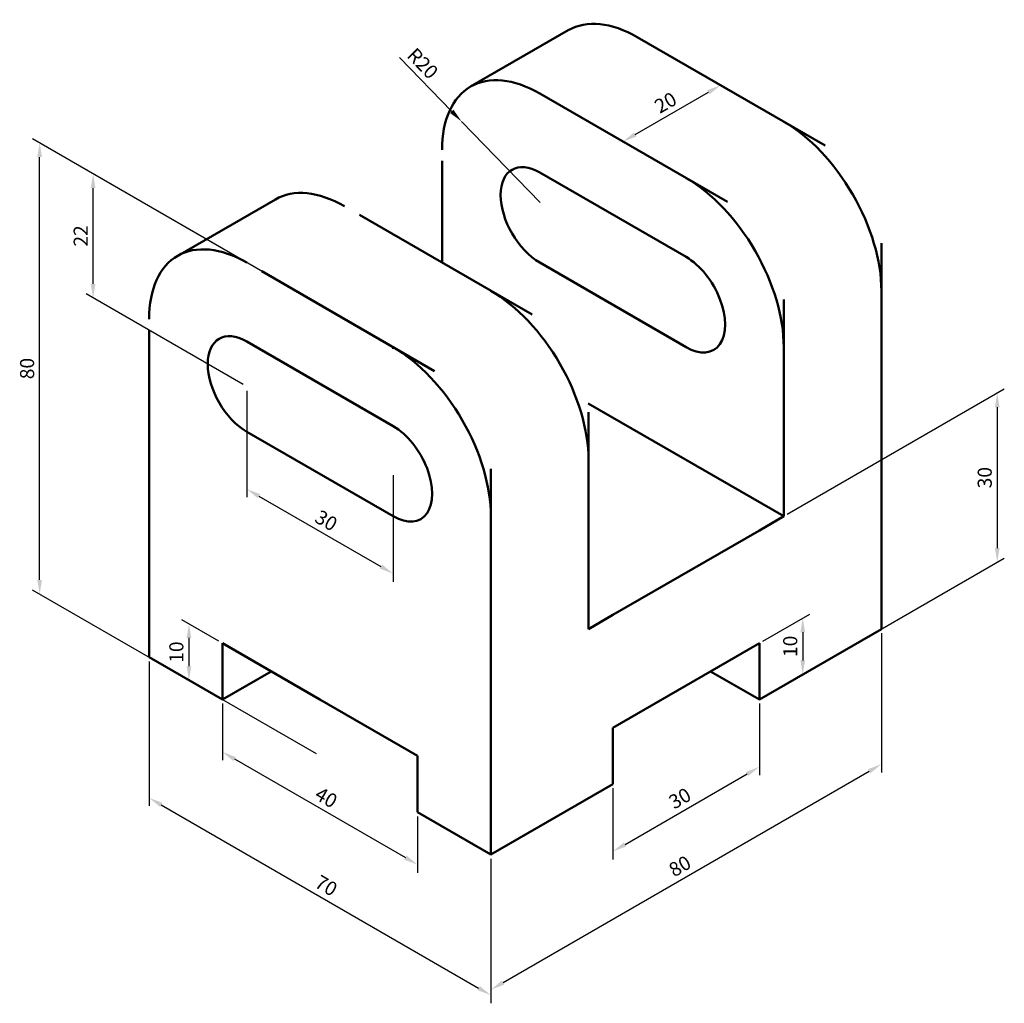
# Model space of a CAD drawing. Units: millimetres. Extents: x 2392 to 2567, y 1870 to 2044.
import ezdxf

# ---------------------------------------------------------------- set-up
doc = ezdxf.new("R2010")
doc.units = ezdxf.units.MM
doc.layers.add('M-DIMS', color=2, linetype='Continuous', lineweight=25)
doc.layers.add('M-OUTL', color=7, linetype='Continuous', lineweight=50)
doc.styles.get("Standard").update_dxf_attribs({"font": 'arial.ttf'})
doc.dimstyles.new('ISO-25', dxfattribs={"dimtxt": 2.5, "dimasz": 2.5, "dimexe": 1.25, "dimexo": 0.625, "dimtad": 1, "dimtxsty": 'Standard', "dimcen": 2.5, "dimadec": 0, "dimazin": 0, "dimtfac": 1, "dimtmove": 0, "dimatfit": 3, "dimfxl": 1, "dimarcsym": 0})

# ---------------------------------------------------------------- blocks, each defined once
blk = doc.blocks.new('*D1')
at = {"layer": 'Defpoints', "color": 0, "transparency": 16777216}
for p in [(2523.54, 1923.45), (2523.54, 1911.51), (2497.56, 1908.45)]:
    blk.add_point(p, dxfattribs=at)
at = {"layer": 'M-DIMS', "color": 0, "lineweight": -2, "transparency": 16777216}
for p, q in [((2523.54, 1922.73), (2523.54, 1910.07)), ((2499.73, 1897.76), (2521.38, 1910.26)), ((2497.56, 1907.73), (2497.56, 1895.07))]:
    blk.add_line(p, q, dxfattribs=at)
at = {"layer": 'M-DIMS', "color": 0, "transparency": 16777216}
for points in [[(2521.17, 1910.62), (2521.58, 1909.9), (2523.54, 1911.51)], [(2499.52, 1898.12), (2499.93, 1897.4), (2497.56, 1896.51)]]:
    blk.add_solid(points, dxfattribs=at)
at = {"layer": 'M-DIMS', "color": 0, "transparency": 16777216, "insert": (2509.6, 1905.66), "char_height": 2.5, "attachment_point": 5, "rotation": 30}
blk.add_mtext('30', dxfattribs=at)
blk = doc.blocks.new('*D2')
at = {"layer": 'Defpoints', "color": 0, "transparency": 16777216}
for p in [(2545.19, 1935.95), (2545.19, 1911.99), (2475.91, 1895.95)]:
    blk.add_point(p, dxfattribs=at)
at = {"layer": 'M-DIMS', "color": 0, "lineweight": -2, "transparency": 16777216}
for p, q in [((2545.19, 1935.23), (2545.19, 1910.54)), ((2478.08, 1873.24), (2543.03, 1910.74)), ((2475.91, 1895.23), (2475.91, 1870.54))]:
    blk.add_line(p, q, dxfattribs=at)
at = {"layer": 'M-DIMS', "color": 0, "transparency": 16777216}
for points in [[(2542.82, 1911.1), (2543.24, 1910.38), (2545.19, 1911.99)], [(2477.87, 1873.6), (2478.28, 1872.88), (2475.91, 1871.99)]]:
    blk.add_solid(points, dxfattribs=at)
at = {"layer": 'M-DIMS', "color": 0, "transparency": 16777216, "insert": (2509.6, 1893.63), "char_height": 2.5, "attachment_point": 5, "rotation": 30}
blk.add_mtext('80', dxfattribs=at)
blk = doc.blocks.new('*D3')
at = {"layer": 'Defpoints', "color": 0, "transparency": 16777216}
for p in [(2428.28, 1923.45), (2462.92, 1903.45), (2462.92, 1894.16)]:
    blk.add_point(p, dxfattribs=at)
at = {"layer": 'M-DIMS', "color": 0, "lineweight": -2, "transparency": 16777216}
for p, q in [((2428.28, 1922.73), (2428.28, 1912.72)), ((2430.44, 1912.91), (2460.75, 1895.41)), ((2462.92, 1902.73), (2462.92, 1892.72))]:
    blk.add_line(p, q, dxfattribs=at)
at = {"layer": 'M-DIMS', "color": 0, "transparency": 16777216}
for points in [[(2430.65, 1913.27), (2430.24, 1912.55), (2428.28, 1914.16)], [(2460.96, 1895.77), (2460.55, 1895.05), (2462.92, 1894.16)]]:
    blk.add_solid(points, dxfattribs=at)
at = {"layer": 'M-DIMS', "color": 0, "transparency": 16777216, "insert": (2446.55, 1905.81), "char_height": 2.5, "attachment_point": 5, "rotation": 330}
blk.add_mtext('40', dxfattribs=at)
blk = doc.blocks.new('*D4')
at = {"layer": 'Defpoints', "color": 0, "transparency": 16777216}
for p in [(2415.29, 1930.95), (2475.91, 1895.95), (2475.91, 1871.02)]:
    blk.add_point(p, dxfattribs=at)
at = {"layer": 'M-DIMS', "color": 0, "lineweight": -2, "transparency": 16777216}
for p, q in [((2415.29, 1930.23), (2415.29, 1904.58)), ((2417.45, 1904.77), (2473.74, 1872.27)), ((2475.91, 1895.23), (2475.91, 1869.58))]:
    blk.add_line(p, q, dxfattribs=at)
at = {"layer": 'M-DIMS', "color": 0, "transparency": 16777216}
for points in [[(2417.66, 1905.13), (2417.24, 1904.41), (2415.29, 1906.02)], [(2473.95, 1872.63), (2473.54, 1871.91), (2475.91, 1871.02)]]:
    blk.add_solid(points, dxfattribs=at)
at = {"layer": 'M-DIMS', "color": 0, "transparency": 16777216, "insert": (2446.55, 1890.17), "char_height": 2.5, "attachment_point": 5, "rotation": 330}
blk.add_mtext('70', dxfattribs=at)
blk = doc.blocks.new('*D5')
at = {"layer": 'Defpoints', "color": 0, "transparency": 16777216}
for p in [(2395.87, 2022.16), (2445.6, 1993.45), (2445.6, 1913.45)]:
    blk.add_point(p, dxfattribs=at)
at = {"layer": 'M-DIMS', "color": 0, "lineweight": -2, "transparency": 16777216}
for p, q in [((2444.97, 1993.81), (2394.62, 2022.88)), ((2395.87, 1944.66), (2395.87, 2019.66)), ((2444.97, 1913.81), (2394.62, 1942.88))]:
    blk.add_line(p, q, dxfattribs=at)
at = {"layer": 'M-DIMS', "color": 0, "transparency": 16777216}
for points in [[(2395.46, 2019.66), (2396.29, 2019.66), (2395.87, 2022.16)], [(2395.46, 1944.66), (2396.29, 1944.66), (2395.87, 1942.16)]]:
    blk.add_solid(points, dxfattribs=at)
at = {"layer": 'M-DIMS', "color": 0, "transparency": 16777216, "insert": (2393.97, 1982.16), "char_height": 2.5, "attachment_point": 5, "rotation": 90}
blk.add_mtext('80', dxfattribs=at)
blk = doc.blocks.new('*D6')
at = {"layer": 'Defpoints', "color": 0, "transparency": 16777216}
for p in [(2405.35, 2016.68), (2432.61, 2000.95), (2432.61, 1978.95)]:
    blk.add_point(p, dxfattribs=at)
at = {"layer": 'M-DIMS', "color": 0, "lineweight": -2, "transparency": 16777216}
for p, q in [((2431.98, 2001.31), (2404.1, 2017.41)), ((2405.35, 1997.18), (2405.35, 2014.18)), ((2431.98, 1979.31), (2404.1, 1995.41))]:
    blk.add_line(p, q, dxfattribs=at)
at = {"layer": 'M-DIMS', "color": 0, "transparency": 16777216}
for points in [[(2404.94, 2014.18), (2405.77, 2014.18), (2405.35, 2016.68)], [(2404.94, 1997.18), (2405.77, 1997.18), (2405.35, 1994.68)]]:
    blk.add_solid(points, dxfattribs=at)
at = {"layer": 'M-DIMS', "color": 0, "transparency": 16777216, "insert": (2403.47, 2005.68), "char_height": 2.5, "attachment_point": 5, "rotation": 90}
blk.add_mtext('22', dxfattribs=at)
blk = doc.blocks.new('*D7')
at = {"layer": 'Defpoints', "color": 0, "transparency": 16777216}
for p in [(2432.61, 1978.95), (2458.59, 1963.95), (2458.59, 1945.78)]:
    blk.add_point(p, dxfattribs=at)
at = {"layer": 'M-DIMS', "color": 0, "lineweight": -2, "transparency": 16777216}
for p, q in [((2432.61, 1978.23), (2432.61, 1959.34)), ((2458.59, 1963.23), (2458.59, 1944.34)), ((2434.77, 1959.53), (2456.42, 1947.03))]:
    blk.add_line(p, q, dxfattribs=at)
at = {"layer": 'M-DIMS', "color": 0, "transparency": 16777216}
for points in [[(2434.98, 1959.89), (2434.57, 1959.17), (2432.61, 1960.78)], [(2456.63, 1947.39), (2456.22, 1946.67), (2458.59, 1945.78)]]:
    blk.add_solid(points, dxfattribs=at)
at = {"layer": 'M-DIMS', "color": 0, "transparency": 16777216, "insert": (2446.55, 1954.93), "char_height": 2.5, "attachment_point": 5, "rotation": 330}
blk.add_mtext('30', dxfattribs=at)
blk = doc.blocks.new('*D8')
at = {"layer": 'Defpoints', "color": 0, "transparency": 16777216}
for p in [(2470.72, 2025.98), (2484.67, 2011.64)]:
    blk.add_point(p, dxfattribs=at)
at = {"layer": 'M-DIMS', "color": 0, "lineweight": -2, "transparency": 16777216}
for p, q in [((2459.71, 2037.31), (2468.98, 2027.78)), ((2484.67, 2011.64), (2470.72, 2025.98))]:
    blk.add_line(p, q, dxfattribs=at)
at = {"layer": 'M-DIMS', "color": 0, "transparency": 16777216}
blk.add_solid([(2469.28, 2028.07), (2468.68, 2027.49), (2470.72, 2025.98)], dxfattribs=at)
at = {"layer": 'M-DIMS', "color": 0, "transparency": 16777216, "insert": (2463.59, 2036.05), "char_height": 2.5, "attachment_point": 5, "rotation": 314.1916}
blk.add_mtext('R20', dxfattribs=at)
blk = doc.blocks.new('*D9')
at = {"layer": 'Defpoints', "color": 0, "transparency": 16777216}
for p in [(2516.67, 2032.42), (2527.87, 2025.95), (2510.55, 2015.95)]:
    blk.add_point(p, dxfattribs=at)
at = {"layer": 'M-DIMS', "color": 0, "lineweight": -2, "transparency": 16777216}
for p, q in [((2527.25, 2026.31), (2515.42, 2033.14)), ((2501.51, 2023.67), (2514.5, 2031.17)), ((2509.93, 2016.31), (2498.1, 2023.14))]:
    blk.add_line(p, q, dxfattribs=at)
at = {"layer": 'M-DIMS', "color": 0, "transparency": 16777216}
for points in [[(2514.29, 2031.53), (2514.71, 2030.81), (2516.67, 2032.42)], [(2501.3, 2024.03), (2501.72, 2023.31), (2499.35, 2022.42)]]:
    blk.add_solid(points, dxfattribs=at)
at = {"layer": 'M-DIMS', "color": 0, "transparency": 16777216, "insert": (2507.06, 2029.06), "char_height": 2.5, "attachment_point": 5, "rotation": 30}
blk.add_mtext('20', dxfattribs=at)
blk = doc.blocks.new('*D10')
at = {"layer": 'Defpoints', "color": 0, "transparency": 16777216}
for p in [(2527.87, 1955.95), (2565.74, 1947.81), (2527.87, 1925.95)]:
    blk.add_point(p, dxfattribs=at)
at = {"layer": 'M-DIMS', "color": 0, "lineweight": -2, "transparency": 16777216}
for p, q in [((2528.5, 1956.31), (2566.99, 1978.54)), ((2565.74, 1975.31), (2565.74, 1950.31)), ((2528.5, 1926.31), (2566.99, 1948.54))]:
    blk.add_line(p, q, dxfattribs=at)
at = {"layer": 'M-DIMS', "color": 0, "transparency": 16777216}
for points in [[(2565.33, 1975.31), (2566.16, 1975.31), (2565.74, 1977.81)], [(2565.33, 1950.31), (2566.16, 1950.31), (2565.74, 1947.81)]]:
    blk.add_solid(points, dxfattribs=at)
at = {"layer": 'M-DIMS', "color": 0, "transparency": 16777216, "insert": (2563.84, 1962.81), "char_height": 2.5, "attachment_point": 5, "rotation": 90}
blk.add_mtext('30', dxfattribs=at)
blk = doc.blocks.new('*D11')
at = {"layer": 'Defpoints', "color": 0, "transparency": 16777216}
for p in [(2523.54, 1933.45), (2531.24, 1927.89), (2523.54, 1923.45)]:
    blk.add_point(p, dxfattribs=at)
at = {"layer": 'M-DIMS', "color": 0, "lineweight": -2, "transparency": 16777216}
for p, q in [((2524.17, 1933.81), (2532.49, 1938.61)), ((2531.24, 1935.39), (2531.24, 1930.39)), ((2524.17, 1923.81), (2532.49, 1928.61))]:
    blk.add_line(p, q, dxfattribs=at)
at = {"layer": 'M-DIMS', "color": 0, "transparency": 16777216}
for points in [[(2530.82, 1935.39), (2531.65, 1935.39), (2531.24, 1937.89)], [(2530.82, 1930.39), (2531.65, 1930.39), (2531.24, 1927.89)]]:
    blk.add_solid(points, dxfattribs=at)
at = {"layer": 'M-DIMS', "color": 0, "transparency": 16777216, "insert": (2529.34, 1932.89), "char_height": 2.5, "attachment_point": 5, "rotation": 90}
blk.add_mtext('10', dxfattribs=at)
blk = doc.blocks.new('*D12')
at = {"layer": 'Defpoints', "color": 0, "transparency": 16777216}
for p in [(2428.28, 1933.45), (2422.36, 1926.87), (2428.28, 1923.45)]:
    blk.add_point(p, dxfattribs=at)
at = {"layer": 'M-DIMS', "color": 0, "lineweight": -2, "transparency": 16777216}
for p, q in [((2427.65, 1933.81), (2421.11, 1937.59)), ((2422.36, 1934.37), (2422.36, 1929.37)), ((2427.65, 1923.81), (2421.11, 1927.59))]:
    blk.add_line(p, q, dxfattribs=at)
at = {"layer": 'M-DIMS', "color": 0, "transparency": 16777216}
for points in [[(2421.94, 1934.37), (2422.77, 1934.37), (2422.36, 1936.87)], [(2421.94, 1929.37), (2422.77, 1929.37), (2422.36, 1926.87)]]:
    blk.add_solid(points, dxfattribs=at)
at = {"layer": 'M-DIMS', "color": 0, "transparency": 16777216, "insert": (2420.45, 1931.87), "char_height": 2.5, "attachment_point": 5, "rotation": 90}
blk.add_mtext('10', dxfattribs=at)

msp = doc.modelspace()

# ---------------------------------------------------------------- linework, layer by layer
at = {"layer": 'M-OUTL'}
for p, q in [((2489.644, 2042.163), (2472.323, 2032.163)), ((2535.192, 2021.723), (2501.891, 2040.95)), ((2517.872, 2011.723), (2484.57, 2030.95)), ((2517.872, 2011.723), (2484.57, 2030.95)), ((2467.25, 2018.987), (2467.25, 2000.95)), ((2484.57, 2016.95), (2510.551, 2001.95)), ((2437.682, 2012.163), (2420.362, 2002.163)), ((2452.583, 2009.417), (2483.23, 1991.723)), ((2545.192, 1935.95), (2545.192, 2004.403)), ((2484.57, 2000.95), (2510.551, 1985.95)), ((2435.263, 1999.417), (2465.91, 1981.723)), ((2527.872, 1955.95), (2527.872, 1994.403)), ((2527.872, 1955.95), (2527.872, 1994.403)), ((2415.288, 1988.95), (2415.288, 1930.95)), ((2432.609, 1986.95), (2458.589, 1971.95)), ((2458.589, 1985.682), (2458.589, 1985.95)), ((2527.872, 1955.95), (2493.168, 1975.986)), ((2493.23, 1974.403), (2493.23, 1935.95)), ((2432.609, 1970.95), (2458.589, 1955.95)), ((2475.91, 1895.95), (2475.91, 1964.403)), ((2523.541, 1953.45), (2527.872, 1955.95)), ((2497.561, 1938.45), (2523.541, 1953.45)), ((2497.561, 1938.45), (2493.23, 1935.95)), ((2523.541, 1923.45), (2545.192, 1935.95)), ((2428.279, 1923.45), (2428.279, 1933.45)), ((2428.279, 1933.45), (2445.599, 1923.45)), ((2510.551, 1925.95), (2523.541, 1933.45)), ((2523.541, 1933.45), (2523.541, 1923.45)), ((2415.288, 1930.95), (2428.279, 1923.45)), ((2428.279, 1923.45), (2436.939, 1928.45)), ((2523.541, 1923.45), (2514.881, 1928.45)), ((2475.91, 1895.95), (2475.91, 1925.95)), ((2510.551, 1925.95), (2497.561, 1918.45)), ((2445.599, 1923.45), (2462.92, 1913.45)), ((2497.561, 1918.45), (2497.561, 1908.45)), ((2462.92, 1913.45), (2462.92, 1903.45)), ((2475.91, 1895.95), (2497.561, 1908.45)), ((2462.92, 1903.45), (2475.91, 1895.95))]:
    msp.add_line(p, q, dxfattribs=at)
for centre, major_axis, start_param, end_param in [((2501.891, 2020.95), (12.247, -21.213), 2.3561944, 3.1415927), ((2484.571, 2010.95), (12.247, -21.213), 2.3561944, 3.1415927), ((2484.571, 2010.95), (12.247, -21.213), 3.1415927, 3.9269909), ((2527.872, 2005.95), (12.247, -21.213), 0.7853981, 2.3561946), ((2484.57, 2008.95), (4.899, -8.485), 2.3561945, 5.4977871), ((2510.551, 1995.95), (12.247, -21.213), 0.7853981, 2.3561946), ((2449.93, 1990.95), (12.247, -21.213), 2.3561944, 3.1415927), ((2432.609, 1980.95), (12.247, -21.213), 2.3561944, 3.1415927), ((2432.609, 1980.95), (12.247, -21.213), 3.1415927, 3.9269909), ((2510.551, 1993.95), (4.899, -8.485), 5.4977871, 8.6393798), ((2475.91, 1975.95), (12.247, -21.213), 0.7853981, 2.3561946), ((2432.609, 1978.95), (4.899, -8.485), 2.3561945, 5.4977871), ((2458.59, 1965.95), (12.247, -21.213), 0.7853981, 2.3561946), ((2458.589, 1963.95), (4.899, -8.485), 5.4977871, 8.6393798)]:
    msp.add_ellipse(centre, major_axis=major_axis, ratio=0.5773503, start_param=start_param, end_param=end_param, dxfattribs=at)

# ---------------------------------------------------------------- dimensions: what is measured, and where the dimension line sits
at = {"layer": 'M-DIMS'}
dim = msp.add_radius_dim(center=(2484.666, 2011.644), mpoint=(2470.725, 2025.985), dimstyle='ISO-25', override={"dimclrd": 0, "dimclre": 0, "dimclrt": 0}, dxfattribs=at)
dim.commit()
dim.dimension.update_dxf_attribs({"geometry": '*D8', "text_midpoint": (2462.228, 2034.724), "dimtype": 164})
for p1, p2, distance, picture, middle in [((2510.551, 2015.95), (2527.872, 2025.95), 11.203, '*D9', (2507.057, 2029.065)), ((2445.599, 1913.45), (2445.599, 1993.45), 49.727, '*D5', (2393.971, 1982.16)), ((2432.609, 1978.95), (2432.609, 2000.95), 27.254, '*D6', (2403.474, 2005.685)), ((2432.609, 1978.95), (2458.589, 1963.95), -15.736, '*D7', (2446.55, 1954.926)), ((2527.872, 1955.95), (2527.872, 1925.95), 37.87, '*D10', (2563.84, 1962.814)), ((2428.279, 1933.45), (2428.279, 1923.45), -5.923, '*D12', (2420.454, 1931.869)), ((2523.541, 1933.45), (2523.541, 1923.45), 7.696, '*D11', (2529.336, 1932.893)), ((2475.91, 1895.95), (2545.192, 1935.95), -20.753, '*D2', (2509.6, 1893.633)), ((2415.288, 1930.95), (2475.91, 1895.95), -21.59, '*D4', (2446.55, 1890.166)), ((2428.279, 1923.45), (2462.92, 1903.45), -8.042, '*D3', (2446.55, 1905.81)), ((2497.561, 1908.45), (2523.541, 1923.45), -10.34, '*D1', (2509.6, 1905.658))]:
    dim = msp.add_aligned_dim(p1=p1, p2=p2, distance=distance, dimstyle='ISO-25', override={"dimclrd": 0, "dimclre": 0, "dimclrt": 0}, dxfattribs=at)
    dim.commit()
    dim.dimension.update_dxf_attribs({"geometry": picture, "text_midpoint": middle})

doc.saveas('drawing.dxf')
